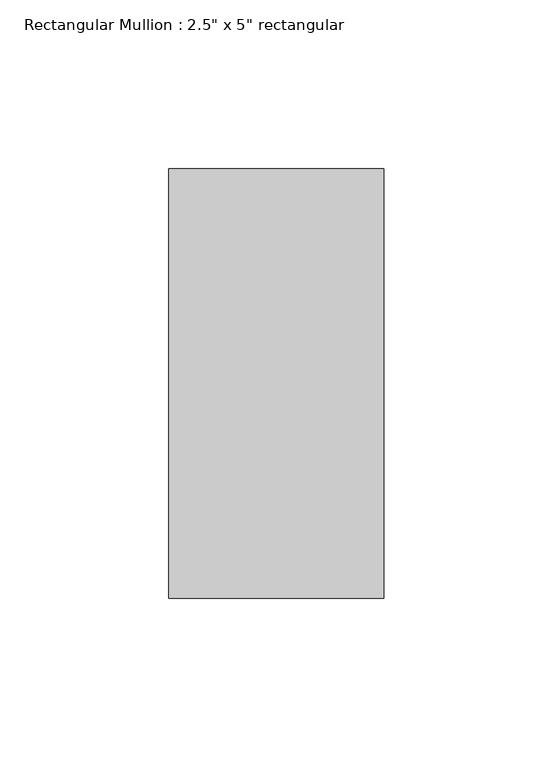
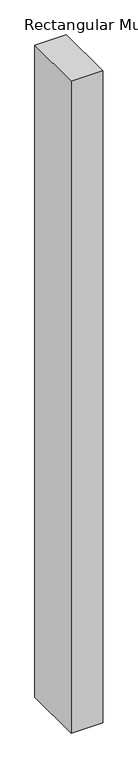
"""IFC4 building model written with IfcOpenShell, lengths in millimetres: member geometry."""

from ifc_helpers import new_model, si_unit, frame, origin, place, context, project, spatial, polyline, outline, extrude, source, transform, mapped, element, save


def member_9fe852e5(model_context):
    return source(origin(), model_context, "Body", "SweptSolid", [
        extrude(outline(polyline([(0.0, 63.5), (0.0, -63.5), (-63.5, -63.5), (-63.5, 63.5), (0.0, 63.5)])), frame((0.0, 0.0, -1391.4079139), z_axis=(0.0, 0.0, 1.0), x_axis=(1.0, 0.0, 0.0)), (0.0, 0.0, 1.0), 1391.4079139),
    ])


if __name__ == "__main__":
    model = new_model("IFC4")
    model_context = context("Model", 3, world=origin())
    ifc_project = project(units=[si_unit("LENGTHUNIT", "METRE", prefix="MILLI")], contexts=[model_context])
    site = spatial("IfcSite", under=ifc_project)
    building = spatial("IfcBuilding", under=site)
    placement = place(None, origin())
    member_shape = member_9fe852e5(model_context)
    element("IfcMember", 1, ObjectType="Rectangular Mullion : 2.5\" x 5\" rectangular", at=placement, inside=building, context=model_context, shape_type="MappedRepresentation", body=[
        mapped(member_shape, transform((0.0, 0.0, 0.0), x_axis=(1.0, 0.0, 0.0), y_axis=(0.0, 1.0, 0.0), z_axis=(0.0, 0.0, 1.0))),
    ])
    save(model, "model.ifc")

# Revit data of these elements
# Type "Rectangular Mullion : 2.5\" x 5\" rectangular"
#   built-in parameter 1007304 = 0.416667 (stored number, unit not read)
#   built-in parameter 1007301 = 0.104167 (stored number, unit not read)
#   built-in parameter 1007300 = 0.104167 (stored number, unit not read)
# Element 1 (IfcMember, "Rectangular Mullion : 2.5\" x 5\" rectangular")
#   Materials on its faces: "Aluminum"
# Materials
#   "Aluminum": class "Metal", colour RGB 247 247 247, transparency 0, Description = "Aluminum 6061", Cost = 0
